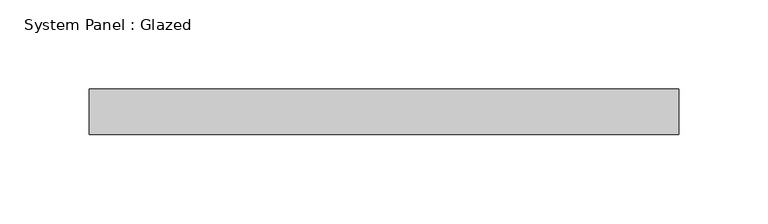
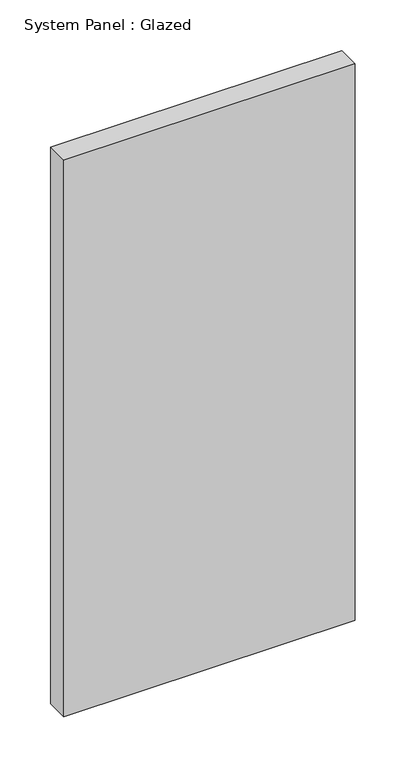
"""IFC4 building model written with IfcOpenShell, lengths in millimetres: plate geometry, System Panel : Glazed."""

from ifc_helpers import new_model, si_unit, origin, origin_with_axes, place, context, project, spatial, polyline, outline, extrude, source, transform, mapped, element, save


def system_panel_glazed_db16a638(model_context):
    return source(origin(), model_context, "Body", "SweptSolid", [
        extrude(outline(polyline([(165.1, 19.05), (-165.1, 19.05), (-165.1, 44.45), (165.1, 44.45), (165.1, 19.05)])), origin_with_axes(), (0.0, 0.0, 1.0), 666.75),
    ])


if __name__ == "__main__":
    model = new_model("IFC4")
    model_context = context("Model", 3, world=origin())
    ifc_project = project(units=[si_unit("LENGTHUNIT", "METRE", prefix="MILLI")], contexts=[model_context])
    site = spatial("IfcSite", under=ifc_project)
    building = spatial("IfcBuilding", under=site)
    placement = place(None, origin())
    system_panel_glazed_shape = system_panel_glazed_db16a638(model_context)
    element("IfcPlate", 1, ObjectType="System Panel : Glazed", at=placement, inside=building, context=model_context, shape_type="MappedRepresentation", body=[
        mapped(system_panel_glazed_shape, transform((0.0, 0.0, 0.0), x_axis=(1.0, 0.0, 0.0), y_axis=(0.0, 1.0, 0.0), z_axis=(0.0, 0.0, 1.0))),
    ])
    save(model, "model.ifc")

# Revit data of these elements
# Type "System Panel : Glazed"
#   Construction Type Id = "GSP4R"
#   Analytic Construction = "1/8 in Pilkington single glazing"
#   Visual Light Transmittance = 0.9
#   Solar Heat Gain Coefficient = 0.86
#   Heat Transfer Coefficient (U) = 1.18115 BTU/(h·ft²·°F)
#   Define Thermal Properties by = 1
# Element 1 (IfcPlate, "System Panel : Glazed")
#   Materials on its faces: "Glass"
# Materials
#   "Glass": class "Glass", colour RGB 0 128 192, transparency 0.75, Description = "Soda Lime Glass", Cost = 0
